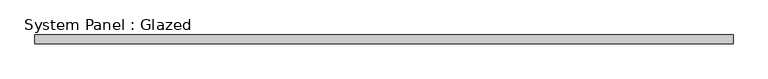
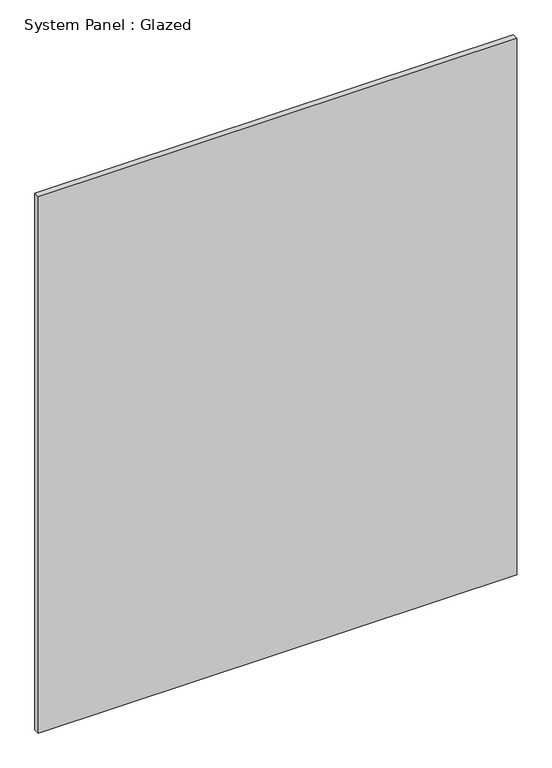
"""IFC4 building model written with IfcOpenShell, lengths in millimetres: plate geometry, System Panel : Glazed."""

from ifc_helpers import new_model, si_unit, origin, origin_with_axes, place, context, project, spatial, polyline, outline, extrude, source, transform, mapped, element, save


def system_panel_glazed_2306c2a7(model_context):
    return source(origin(), model_context, "Body", "SweptSolid", [
        extrude(outline(polyline([(1018.1166667, 19.05), (-1018.1166667, 19.05), (-1018.1166667, 44.45), (1018.1166667, 44.45), (1018.1166667, 19.05)])), origin_with_axes(), (0.0, 0.0, 1.0), 2413.0),
    ])


if __name__ == "__main__":
    model = new_model("IFC4")
    model_context = context("Model", 3, world=origin())
    ifc_project = project(units=[si_unit("LENGTHUNIT", "METRE", prefix="MILLI")], contexts=[model_context])
    site = spatial("IfcSite", under=ifc_project)
    building = spatial("IfcBuilding", under=site)
    placement = place(None, origin())
    system_panel_glazed_shape = system_panel_glazed_2306c2a7(model_context)
    element("IfcPlate", 1, ObjectType="System Panel : Glazed", at=placement, inside=building, context=model_context, shape_type="MappedRepresentation", body=[
        mapped(system_panel_glazed_shape, transform((0.0, 0.0, 0.0), x_axis=(1.0, 0.0, 0.0), y_axis=(0.0, 1.0, 0.0), z_axis=(0.0, 0.0, 1.0))),
    ])
    save(model, "model.ifc")

# Revit data of these elements
# Type "System Panel : Glazed"
#   Construction Type Id = "GSP4R"
#   Analytic Construction = "1/8 in Pilkington single glazing"
#   Visual Light Transmittance = 0.9
#   Solar Heat Gain Coefficient = 0.86
#   Heat Transfer Coefficient (U) = 1.18115 BTU/(h·ft²·°F)
# Element 1 (IfcPlate, "System Panel : Glazed")
#   Materials on its faces: "Glass"
# Materials
#   "Glass": class "Glass", colour RGB 0 128 192, transparency 0.75, Description = "Soda Lime Glass", Cost = 0
